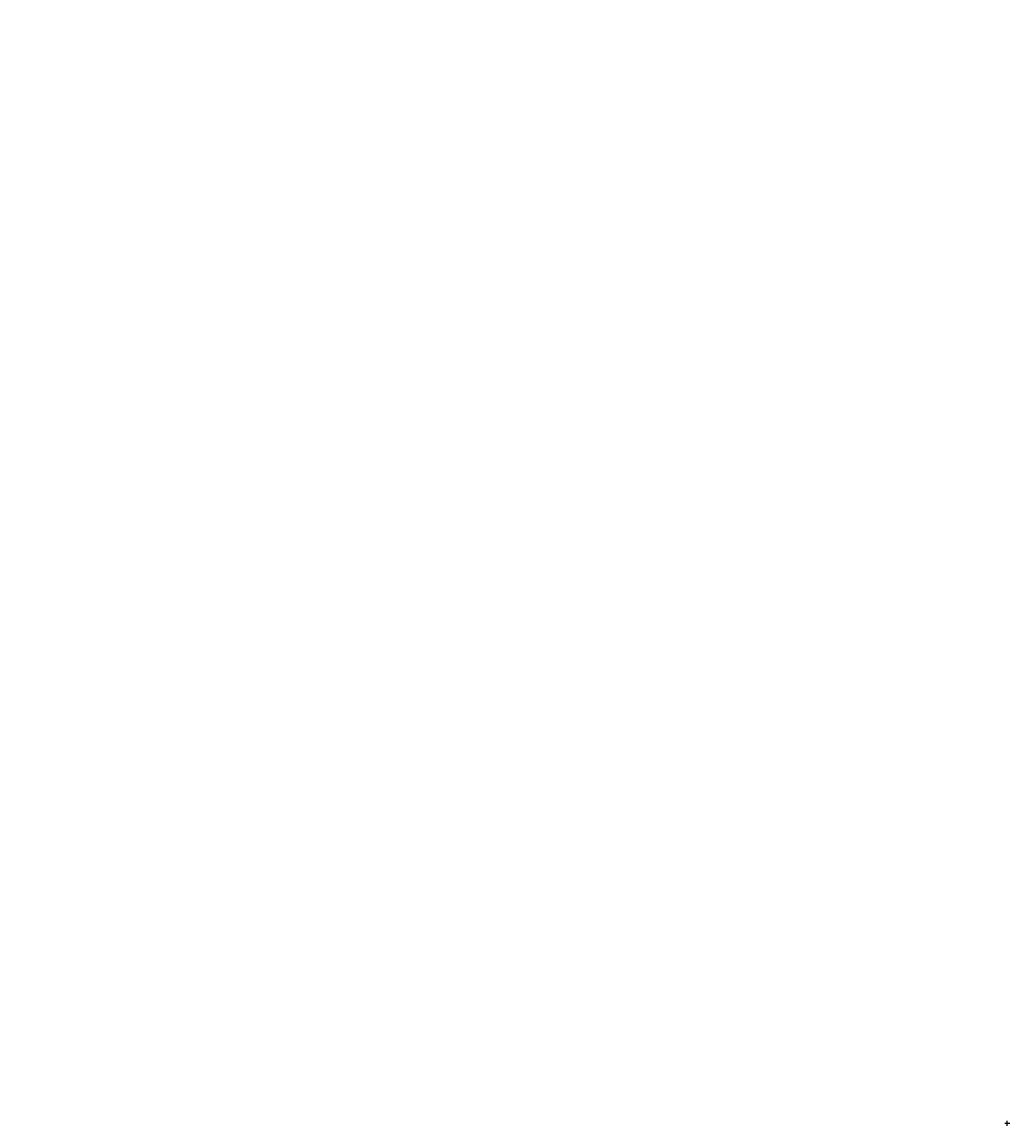
# Model space of a CAD drawing. Units: inches. Extents: x 114 to 236, y -51 to 115.
# Tile 1 of 14: x 146 to 180, y -51 to -13. Entities that reach past the tile are written whole.
import ezdxf

# ---------------------------------------------------------------- set-up
doc = ezdxf.new("R2010")
doc.units = ezdxf.units.IN
doc.header["$MEASUREMENT"] = 0
doc.layers.add('M-DIMS', color=2, linetype='Continuous', lineweight=18)
doc.styles.get("Standard").update_dxf_attribs({"font": 'arial.ttf'})
doc.dimstyles.get("Standard").update_dxf_attribs({"dimtxt": 0.18, "dimasz": 0.18, "dimexe": 0.18, "dimexo": 0.0625, "dimgap": 0.09, "dimtad": 0, "dimtih": 1, "dimtoh": 1, "dimdec": 4, "dimzin": 0, "dimdsep": 46, "dimtxsty": 'Standard', "dimcen": 0.09, "dimadec": 0, "dimazin": 0, "dimtfac": 1, "dimtdec": 4, "dimtofl": 0, "dimtmove": 0, "dimatfit": 3, "dimfxl": 1, "dimtolj": 1, "dimtzin": 0, "dimarcsym": 0})

# ---------------------------------------------------------------- blocks, each defined once
blk = doc.blocks.new('*D14')
at = {"layer": 'Defpoints', "color": 0, "transparency": 16777216}
for p in [(159.689, 5.682), (180.229, -50.693)]:
    blk.add_point(p, dxfattribs=at)
at = {"layer": 'M-DIMS', "color": 0, "lineweight": -2, "transparency": 16777216}
for p, q in [((147.185, 39.507), (147.365, 39.507)), ((147.365, 39.507), (159.627, 5.851)), ((180.139, -50.693), (180.319, -50.693)), ((180.229, -50.783), (180.229, -50.603))]:
    blk.add_line(p, q, dxfattribs=at)
at = {"layer": 'M-DIMS', "color": 0, "transparency": 16777216}
blk.add_solid([(159.655, 5.861), (159.599, 5.841), (159.689, 5.682)], dxfattribs=at)
at = {"layer": 'M-DIMS', "color": 0, "transparency": 16777216, "insert": (146.685, 39.507), "char_height": 0.18, "attachment_point": 5}
blk.add_mtext('\\A1;2X R60', dxfattribs=at)

msp = doc.modelspace()

# ---------------------------------------------------------------- dimensions: what is measured, and where the dimension line sits
at = {"layer": 'M-DIMS'}
dim = msp.add_radius_dim(center=(180.229, -50.693), mpoint=(159.689, 5.682), text='2X <>', dimstyle='Standard', override={"dimdec": 0, "dimlfac": 1, "dimrnd": 0, "dimzin": 0, "dimdsep": 46, "dimlunit": 2}, dxfattribs=at)
dim.commit()
dim.dimension.update_dxf_attribs({"geometry": '*D14', "text_midpoint": (146.685, 39.507), "dimtype": 164})

doc.saveas('drawing.dxf')
